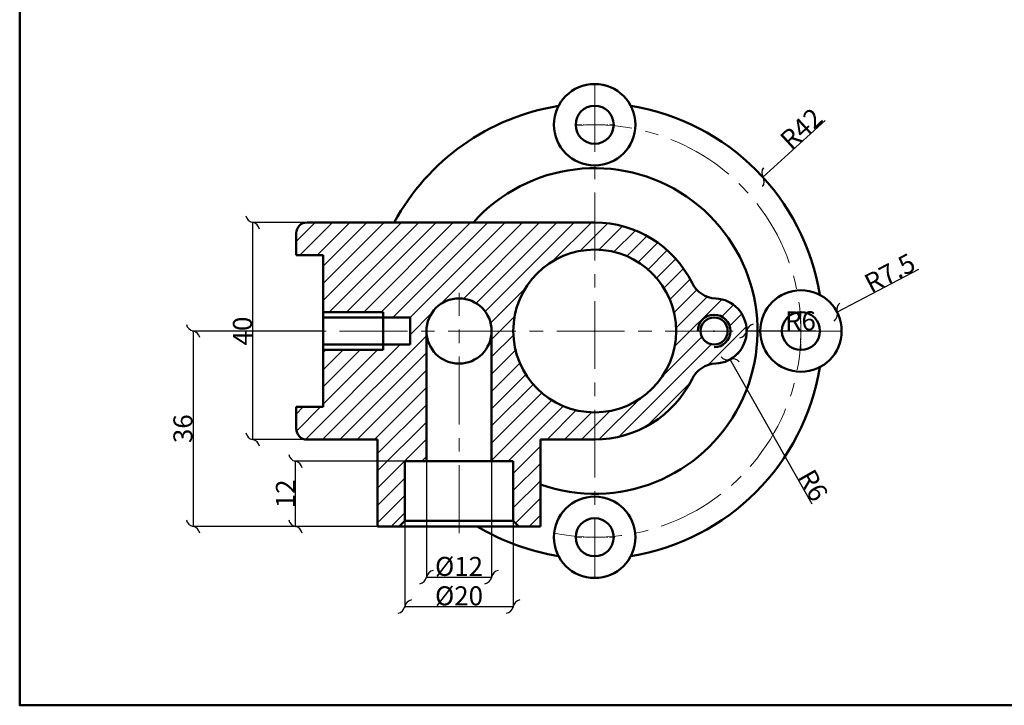
# Model space of a CAD drawing. Units: millimetres. Extents: x 10 to 373, y 9 to 285.
# Tile 1 of 3: x 10 to 191, y 9 to 135. Entities that reach past the tile are written whole.
import ezdxf

# ---------------------------------------------------------------- set-up
doc = ezdxf.new("R2010")
doc.units = ezdxf.units.MM
doc.header["$MEASUREMENT"] = 0
doc.linetypes.add('CENTER', pattern=[2, 1.25, -0.25, 0.25, -0.25])
for name, color, linetype, lineweight in [('M-CNTR', 1, 'CENTER', 18), ('M-DIMS', 2, 'Continuous', 25), ('M-HATC', 8, 'Continuous', 18), ('M-OUTL', 7, 'Continuous', 50), ('M-TTLB', 7, 'Continuous', 50)]:
    doc.layers.add(name, color=color, linetype=linetype, lineweight=lineweight)
doc.styles.get("Standard").update_dxf_attribs({"font": 'arial.ttf'})
doc.dimstyles.get("Standard").update_dxf_attribs({"dimtxt": 3.5, "dimasz": 3.5, "dimexe": 0.18, "dimexo": 0.0625, "dimgap": 0.09, "dimtad": 1, "dimdec": 0, "dimzin": 0, "dimdsep": 46, "dimtxsty": 'Standard', "dimblk": 'INTEGRAL', "dimcen": 0.09, "dimclre": 251, "dimadec": 0, "dimazin": 0, "dimtfac": 1, "dimtdec": 0, "dimtofl": 0, "dimtmove": 0, "dimatfit": 3, "dimfxl": 1, "dimtolj": 1, "dimtzin": 0, "dimarcsym": 0})

# ---------------------------------------------------------------- blocks, each defined once
blk = doc.blocks.new('*U17')
at = {"layer": 'M-CNTR', "color": 0, "transparency": 16777216}
for p, q in [((0, 0.7), (0, 3.62)), ((-3.62, 0), (-0.7, 0)), ((0.7, 0), (3.62, 0)), ((0, -3.62), (0, -0.7))]:
    blk.add_line(p, q, dxfattribs=at)
at = {"layer": 'M-CNTR', "color": 0, "linetype": 'Continuous', "transparency": 16777216}
for p, q in [((-0.35, 0), (0.35, 0)), ((0, -0.35), (0, 0.35))]:
    blk.add_line(p, q, dxfattribs=at)
blk = doc.blocks.new('*U18')
at = {"layer": 'M-CNTR', "color": 0, "transparency": 16777216}
for p, q in [((0, 0.7), (0, 3.62)), ((-3.62, 0), (-0.7, 0)), ((0.7, 0), (3.62, 0)), ((0, -3.62), (0, -0.7))]:
    blk.add_line(p, q, dxfattribs=at)
at = {"layer": 'M-CNTR', "color": 0, "linetype": 'Continuous', "transparency": 16777216}
for p, q in [((-0.35, 0), (0.35, 0)), ((0, -0.35), (0, 0.35))]:
    blk.add_line(p, q, dxfattribs=at)
blk = doc.blocks.new('*U19')
at = {"layer": 'M-CNTR', "color": 0, "transparency": 16777216}
for p, q in [((0, 0.7), (0, 3.62)), ((-3.62, 0), (-0.7, 0)), ((0.7, 0), (3.62, 0)), ((0, -3.62), (0, -0.7))]:
    blk.add_line(p, q, dxfattribs=at)
at = {"layer": 'M-CNTR', "color": 0, "linetype": 'Continuous', "transparency": 16777216}
for p, q in [((-0.35, 0), (0.35, 0)), ((0, -0.35), (0, 0.35))]:
    blk.add_line(p, q, dxfattribs=at)
blk = doc.blocks.new('_Integral')
at = {"color": 0, "linetype": 'ByBlock', "lineweight": -2}
for centre, start, end in [((0.445, -0.091), 102, 168), ((-0.445, 0.091), 282, 348)]:
    blk.add_arc(centre, 0.454, start, end, dxfattribs=at)
blk = doc.blocks.new('*D57')
at = {"layer": 'Defpoints', "color": 0, "transparency": 16777216}
for p in [(52.86, 97.76), (65.25, 97.76), (65.25, 57.76)]:
    blk.add_point(p, dxfattribs=at)
at = {"layer": 'M-DIMS', "color": 0, "lineweight": -2, "transparency": 16777216}
for p, q in [((65.19, 97.76), (52.68, 97.76)), ((52.86, 57.76), (52.86, 97.76)), ((65.19, 57.76), (52.68, 57.76))]:
    blk.add_line(p, q, dxfattribs=at)
at = {"layer": 'M-DIMS', "color": 0, "lineweight": -2, "transparency": 16777216, "xscale": 3.5, "yscale": 3.5, "zscale": 3.5}
for p, rotation in [((52.86, 97.76), 90), ((52.86, 57.76), 270)]:
    blk.add_blockref('_Integral', p, dxfattribs=dict(at, rotation=rotation))
at = {"layer": 'M-DIMS', "color": 0, "transparency": 16777216, "insert": (50.98, 77.76), "char_height": 3.5, "attachment_point": 5, "rotation": 90}
blk.add_mtext('\\A1;40', dxfattribs=at)
blk = doc.blocks.new('*D58')
at = {"layer": 'Defpoints', "color": 0, "transparency": 16777216}
for p in [(65.88, 77.76), (41.89, 41.76), (75.88, 41.76)]:
    blk.add_point(p, dxfattribs=at)
at = {"layer": 'M-DIMS', "color": 0, "lineweight": -2, "transparency": 16777216}
for p, q in [((65.82, 77.76), (41.71, 77.76)), ((41.89, 77.76), (41.89, 41.76)), ((75.82, 41.76), (41.71, 41.76))]:
    blk.add_line(p, q, dxfattribs=at)
at = {"layer": 'M-DIMS', "color": 0, "lineweight": -2, "transparency": 16777216, "xscale": 3.5, "yscale": 3.5, "zscale": 3.5}
for p, rotation in [((41.89, 77.76), 90), ((41.89, 41.76), 270)]:
    blk.add_blockref('_Integral', p, dxfattribs=dict(at, rotation=rotation))
at = {"layer": 'M-DIMS', "color": 0, "transparency": 16777216, "insert": (40.01, 59.76), "char_height": 3.5, "attachment_point": 5, "rotation": 90}
blk.add_mtext('\\A1;36', dxfattribs=at)
blk = doc.blocks.new('*D59')
at = {"layer": 'Defpoints', "color": 0, "transparency": 16777216}
for p in [(60.73, 53.76), (80.88, 53.76), (75.88, 41.76)]:
    blk.add_point(p, dxfattribs=at)
at = {"layer": 'M-DIMS', "color": 0, "lineweight": -2, "transparency": 16777216}
for p, q in [((80.82, 53.76), (60.55, 53.76)), ((60.73, 41.76), (60.73, 53.76)), ((75.82, 41.76), (60.55, 41.76))]:
    blk.add_line(p, q, dxfattribs=at)
at = {"layer": 'M-DIMS', "color": 0, "lineweight": -2, "transparency": 16777216, "xscale": 3.5, "yscale": 3.5, "zscale": 3.5}
for p, rotation in [((60.73, 53.76), 90), ((60.73, 41.76), 270)]:
    blk.add_blockref('_Integral', p, dxfattribs=dict(at, rotation=rotation))
at = {"layer": 'M-DIMS', "color": 0, "transparency": 16777216, "insert": (58.89, 47.76), "char_height": 3.5, "attachment_point": 5, "rotation": 90}
blk.add_mtext('\\A1;12', dxfattribs=at)
blk = doc.blocks.new('*D60')
at = {"layer": 'Defpoints', "color": 0, "transparency": 16777216}
for p in [(80.88, 42.76), (100.88, 42.76), (100.88, 27)]:
    blk.add_point(p, dxfattribs=at)
at = {"layer": 'M-DIMS', "color": 0, "lineweight": -2, "transparency": 16777216}
for p, q in [((80.88, 42.7), (80.88, 26.82)), ((100.88, 42.7), (100.88, 26.82)), ((80.88, 27), (100.88, 27))]:
    blk.add_line(p, q, dxfattribs=at)
at = {"layer": 'M-DIMS', "color": 0, "lineweight": -2, "transparency": 16777216, "xscale": 3.5, "yscale": 3.5, "zscale": 3.5, "rotation": 180}
blk.add_blockref('_Integral', (80.88, 27), dxfattribs=at)
at = {"layer": 'M-DIMS', "color": 0, "lineweight": -2, "transparency": 16777216, "xscale": 3.5, "yscale": 3.5, "zscale": 3.5}
blk.add_blockref('_Integral', (100.88, 27), dxfattribs=at)
at = {"layer": 'M-DIMS', "color": 0, "transparency": 16777216, "insert": (90.88, 28.97), "char_height": 3.5, "attachment_point": 5}
blk.add_mtext('\\A1;%%C20', dxfattribs=at)
blk = doc.blocks.new('*D61')
at = {"layer": 'Defpoints', "color": 0, "transparency": 16777216}
for p in [(84.88, 53.76), (96.88, 53.76), (96.88, 32.42)]:
    blk.add_point(p, dxfattribs=at)
at = {"layer": 'M-DIMS', "color": 0, "lineweight": -2, "transparency": 16777216}
for p, q in [((84.88, 53.7), (84.88, 32.24)), ((96.88, 53.7), (96.88, 32.24)), ((84.88, 32.42), (96.88, 32.42))]:
    blk.add_line(p, q, dxfattribs=at)
at = {"layer": 'M-DIMS', "color": 0, "lineweight": -2, "transparency": 16777216, "xscale": 3.5, "yscale": 3.5, "zscale": 3.5, "rotation": 180}
blk.add_blockref('_Integral', (84.88, 32.42), dxfattribs=at)
at = {"layer": 'M-DIMS', "color": 0, "lineweight": -2, "transparency": 16777216, "xscale": 3.5, "yscale": 3.5, "zscale": 3.5}
blk.add_blockref('_Integral', (96.88, 32.42), dxfattribs=at)
at = {"layer": 'M-DIMS', "color": 0, "transparency": 16777216, "insert": (90.88, 34.39), "char_height": 3.5, "attachment_point": 5}
blk.add_mtext('\\A1;%%C12', dxfattribs=at)
blk = doc.blocks.new('*D62')
at = {"layer": 'Defpoints', "color": 0, "transparency": 16777216}
for p in [(146.89, 106.1), (115.88, 77.76)]:
    blk.add_point(p, dxfattribs=at)
at = {"layer": 'M-DIMS', "color": 0, "lineweight": -2, "transparency": 16777216}
for p, q in [((158.33, 116.56), (146.89, 106.1)), ((115.79, 77.76), (115.97, 77.76)), ((115.88, 77.67), (115.88, 77.85))]:
    blk.add_line(p, q, dxfattribs=at)
at = {"layer": 'M-DIMS', "color": 0, "lineweight": -2, "transparency": 16777216, "xscale": 3.5, "yscale": 3.5, "zscale": 3.5, "rotation": 222.4298559796498}
blk.add_blockref('_Integral', (146.89, 106.1), dxfattribs=at)
at = {"layer": 'M-DIMS', "color": 0, "transparency": 16777216, "insert": (153.95, 115.05), "char_height": 3.5, "attachment_point": 5, "rotation": 42.4299}
blk.add_mtext('\\A1;R42', dxfattribs=at)
blk = doc.blocks.new('*D63')
at = {"layer": 'Defpoints', "color": 0, "transparency": 16777216}
for p in [(160.53, 81.25), (153.88, 77.76)]:
    blk.add_point(p, dxfattribs=at)
at = {"layer": 'M-DIMS', "color": 0, "lineweight": -2, "transparency": 16777216}
for p, q in [((175.52, 89.11), (160.53, 81.25)), ((153.79, 77.76), (153.97, 77.76)), ((153.88, 77.67), (153.88, 77.85))]:
    blk.add_line(p, q, dxfattribs=at)
at = {"layer": 'M-DIMS', "color": 0, "lineweight": -2, "transparency": 16777216, "xscale": 3.5, "yscale": 3.5, "zscale": 3.5, "rotation": 207.6880472213074}
blk.add_blockref('_Integral', (160.53, 81.25), dxfattribs=at)
at = {"layer": 'M-DIMS', "color": 0, "transparency": 16777216, "insert": (170.25, 88.46), "char_height": 3.5, "attachment_point": 5, "rotation": 27.688}
blk.add_mtext('\\A1;R7.5', dxfattribs=at)
blk = doc.blocks.new('*D64')
at = {"layer": 'Defpoints', "color": 0, "transparency": 16777216}
for p in [(137.88, 77.76), (140.84, 72.54)]:
    blk.add_point(p, dxfattribs=at)
at = {"layer": 'M-DIMS', "color": 0, "lineweight": -2, "transparency": 16777216}
for p, q in [((137.79, 77.76), (137.97, 77.76)), ((137.88, 77.67), (137.88, 77.85)), ((155.93, 45.87), (140.84, 72.54))]:
    blk.add_line(p, q, dxfattribs=at)
at = {"layer": 'M-DIMS', "color": 0, "lineweight": -2, "transparency": 16777216, "xscale": 3.5, "yscale": 3.5, "zscale": 3.5, "rotation": 119.5049424371252}
blk.add_blockref('_Integral', (140.84, 72.54), dxfattribs=at)
at = {"layer": 'M-DIMS', "color": 0, "transparency": 16777216, "insert": (156.13, 49.33), "char_height": 3.5, "attachment_point": 5, "rotation": 299.5049}
blk.add_mtext('\\A1;R6', dxfattribs=at)
blk = doc.blocks.new('*D68')
at = {"layer": 'Defpoints', "color": 0, "transparency": 16777216}
for p in [(137.88, 77.76), (143.88, 77.76)]:
    blk.add_point(p, dxfattribs=at)
at = {"layer": 'M-DIMS', "color": 251, "lineweight": -2, "transparency": 16777216}
for p, q in [((137.79, 77.76), (137.97, 77.76)), ((137.88, 77.67), (137.88, 77.85))]:
    blk.add_line(p, q, dxfattribs=at)
at = {"layer": 'M-DIMS', "color": 0, "lineweight": -2, "transparency": 16777216}
blk.add_line((156.71, 77.76), (143.88, 77.76), dxfattribs=at)
at = {"layer": 'M-DIMS', "color": 0, "lineweight": -2, "transparency": 16777216, "xscale": 3.5, "yscale": 3.5, "zscale": 3.5, "rotation": 180.0041921411934}
blk.add_blockref('_Integral', (143.88, 77.76), dxfattribs=at)
at = {"layer": 'M-DIMS', "color": 0, "transparency": 16777216, "insert": (153.8, 79.64), "char_height": 3.5, "attachment_point": 5, "rotation": 0.0042}
blk.add_mtext('\\A1;R6', dxfattribs=at)

msp = doc.modelspace()

# ---------------------------------------------------------------- hatches: boundary and pattern name
at = {"layer": 'M-HATC'}
h = msp.add_hatch(dxfattribs=at)
h.set_pattern_fill('ANSI31', color=256, scale=18)
h.set_pattern_definition([(45, (-376.4816, -107.6296), (-1.59099, 1.59099), [])])
h.paths.add_polyline_path([(84.88, 77.76), (81.88, 77.76), (81.88, 75.26), (76.88, 75.26), (76.88, 74.26), (65.88, 74.26), (65.88, 63.76), (60.88, 63.76), (60.88, 59.76, 0.414214), (62.88, 57.76), (75.88, 57.76), (75.88, 41.76), (79.88, 41.76), (80.88, 42.76), (80.88, 53.76), (84.88, 53.76)])
h.paths.add_polyline_path([(115.88, 92.76), (115.88, 97.76), (62.88, 97.76, 0.414214), (60.88, 95.76), (60.88, 91.76), (65.88, 91.76), (65.88, 81.26), (76.88, 81.26), (76.88, 80.26), (81.88, 80.26), (81.88, 77.76), (84.88, 77.76, -1), (96.88, 77.76), (100.88, 77.76, -0.414214)])
h.paths.add_polyline_path([(100.88, 77.76), (96.88, 77.76), (96.88, 53.76), (100.88, 53.76), (100.88, 42.76), (101.88, 41.76), (105.88, 41.76), (105.88, 57.76), (115.88, 57.76), (115.88, 62.76, -0.414214)])
h.paths.add_polyline_path([(138.18, 83.75, -0.271862), (133.81, 86.62, 0.285332), (115.88, 97.76), (115.88, 92.76, -0.414214), (130.88, 77.76), (134.88, 77.76, -1), (140.88, 77.76), (143.88, 77.76, 0.399643)])
h.paths.add_polyline_path([(143.88, 77.76), (140.88, 77.76), (140.38, 77.76, -1), (135.38, 77.76), (130.88, 77.76, -0.414214), (115.88, 62.76), (115.88, 57.76, 0.285332), (133.81, 68.9, -0.271862), (138.18, 71.77, 0.399643)])

# ---------------------------------------------------------------- linework, layer by layer
at = {"layer": 'M-CNTR', "ltscale": 10}
for p, q in [((115.88, 123.26), (115.88, 32.26)), ((90.88, 40.54), (90.88, 84.8)), ((161.38, 77.76), (65.88, 77.76))]:
    msp.add_line(p, q, dxfattribs=at)
msp.add_arc((115.88, 77.76), 38, 258.6732, 95.2791, dxfattribs=at)
at = {"layer": 'M-OUTL'}
for p, q in [((62.88, 97.76), (115.88, 97.76)), ((60.88, 91.76), (60.88, 95.76)), ((60.88, 91.76), (65.88, 91.76)), ((65.88, 91.76), (65.88, 63.76)), ((65.88, 81.26), (76.88, 81.26)), ((65.88, 80.26), (81.88, 80.26)), ((76.88, 81.26), (76.88, 74.26)), ((81.88, 80.26), (81.88, 75.26)), ((84.88, 53.76), (84.88, 77.76)), ((96.88, 53.76), (96.88, 77.76)), ((65.88, 75.26), (81.88, 75.26)), ((65.88, 74.26), (76.88, 74.26)), ((60.88, 59.76), (60.88, 63.76)), ((60.88, 63.76), (65.88, 63.76)), ((62.88, 57.76), (75.88, 57.76)), ((75.88, 57.76), (75.88, 41.76)), ((105.88, 41.76), (105.88, 57.76)), ((105.88, 57.76), (115.88, 57.76)), ((80.88, 53.76), (100.88, 53.76)), ((80.88, 53.76), (80.88, 42.76)), ((100.88, 53.76), (100.88, 42.76)), ((75.88, 41.76), (105.88, 41.76)), ((79.88, 41.76), (80.88, 42.76)), ((100.88, 42.76), (80.88, 42.76)), ((100.88, 42.76), (101.88, 41.76))]:
    msp.add_line(p, q, dxfattribs=at)
for centre, radius in [((115.88, 115.76), 7.5), ((115.88, 115.76), 3.5), ((115.88, 77.76), 15), ((90.88, 77.76), 6), ((153.88, 77.76), 7.5), ((137.88, 77.76), 2.5), ((153.88, 77.76), 3.5), ((115.88, 39.76), 7.5), ((115.88, 39.76), 3.5)]:
    msp.add_circle(centre, radius, dxfattribs=at)
for centre, radius, start, end in [((115.88, 77.76), 42, 99.1085, 151.5631), ((115.88, 77.76), 42, 9.1085, 80.8915), ((115.88, 77.76), 30, 250.5288, 138.1897), ((62.88, 95.76), 2, 90, 180), ((115.88, 77.76), 20, 26.2993, 90), ((138.44, 88.91), 5.16, 206.2993, 267.1351), ((137.88, 77.76), 6, 272.8649, 87.1351), ((137.88, 77.76), 3, 270, 180), ((115.88, 77.76), 42, 279.1085, 350.8915), ((138.44, 66.61), 5.16, 92.8649, 153.7007), ((115.88, 77.76), 20, 270, 333.7007), ((62.88, 59.76), 2, 180, 270), ((115.88, 77.76), 42, 238.9973, 260.8915)]:
    msp.add_arc(centre, radius, start, end, dxfattribs=at)
at = {"layer": 'M-TTLB'}
msp.add_lwpolyline([(9.93, 285.37), (372.77, 285.37), (372.77, 8.8), (9.93, 8.8)], close=True, dxfattribs=at)

# ---------------------------------------------------------------- block references
at = {"layer": 'M-CNTR'}
for name, p in [('*U17', (115.88, 115.76)), ('*U18', (153.88, 77.76)), ('*U19', (115.88, 39.76))]:
    msp.add_blockref(name, p, dxfattribs=at)

# ---------------------------------------------------------------- dimensions: what is measured, and where the dimension line sits
at = {"layer": 'M-DIMS'}
for center, mpoint, override, picture, middle in [((115.88, 77.76), (146.89, 106.1), {"dimclrd": 0, "dimclre": 0, "dimclrt": 0}, '*D62', (153.95, 115.05)), ((153.88, 77.76), (160.53, 81.25), {"dimdec": 1, "dimclrd": 0, "dimclre": 0, "dimclrt": 0}, '*D63', (170.25, 88.46)), ((137.88, 77.76), (143.88, 77.76), {"dimdec": 0, "dimlfac": 1, "dimrnd": 0, "dimzin": 0, "dimdsep": 46, "dimlunit": 2}, '*D68', (153.8, 79.64))]:
    dim = msp.add_radius_dim(center=center, mpoint=mpoint, dimstyle='Standard', override=override, dxfattribs=at)
    dim.commit()
    dim.dimension.update_dxf_attribs({"geometry": picture, "text_midpoint": middle})
for base, p1, p2, picture, middle in [((52.86, 97.76), (65.25, 57.76), (65.25, 97.76), '*D57', (50.98, 77.76)), ((41.89, 41.76), (65.88, 77.76), (75.88, 41.76), '*D58', (40.01, 59.76)), ((60.73, 53.76), (75.88, 41.76), (80.88, 53.76), '*D59', (58.89, 47.76))]:
    dim = msp.add_linear_dim(base=base, p1=p1, p2=p2, angle=90, dimstyle='Standard', override={"dimclrd": 0, "dimclre": 0, "dimclrt": 0}, dxfattribs=at)
    dim.commit()
    dim.dimension.update_dxf_attribs({"geometry": picture, "text_midpoint": middle})
dim = msp.add_radius_dim(center=(137.88, 77.76), mpoint=(140.84, 72.54), dimstyle='Standard', override={"dimclrd": 0, "dimclre": 0, "dimclrt": 0}, dxfattribs=at)
dim.commit()
dim.dimension.update_dxf_attribs({"geometry": '*D64', "text_midpoint": (154.5, 48.41), "dimtype": 164})
for base, p1, p2, picture, middle in [((96.88, 32.42), (84.88, 53.76), (96.88, 53.76), '*D61', (90.88, 34.39)), ((100.88, 27), (80.88, 42.76), (100.88, 42.76), '*D60', (90.88, 28.97))]:
    dim = msp.add_linear_dim(base=base, p1=p1, p2=p2, text='%%C<>', dimstyle='Standard', override={"dimclrd": 0, "dimclre": 0, "dimclrt": 0}, dxfattribs=at)
    dim.commit()
    dim.dimension.update_dxf_attribs({"geometry": picture, "text_midpoint": middle})

doc.saveas('drawing.dxf')
